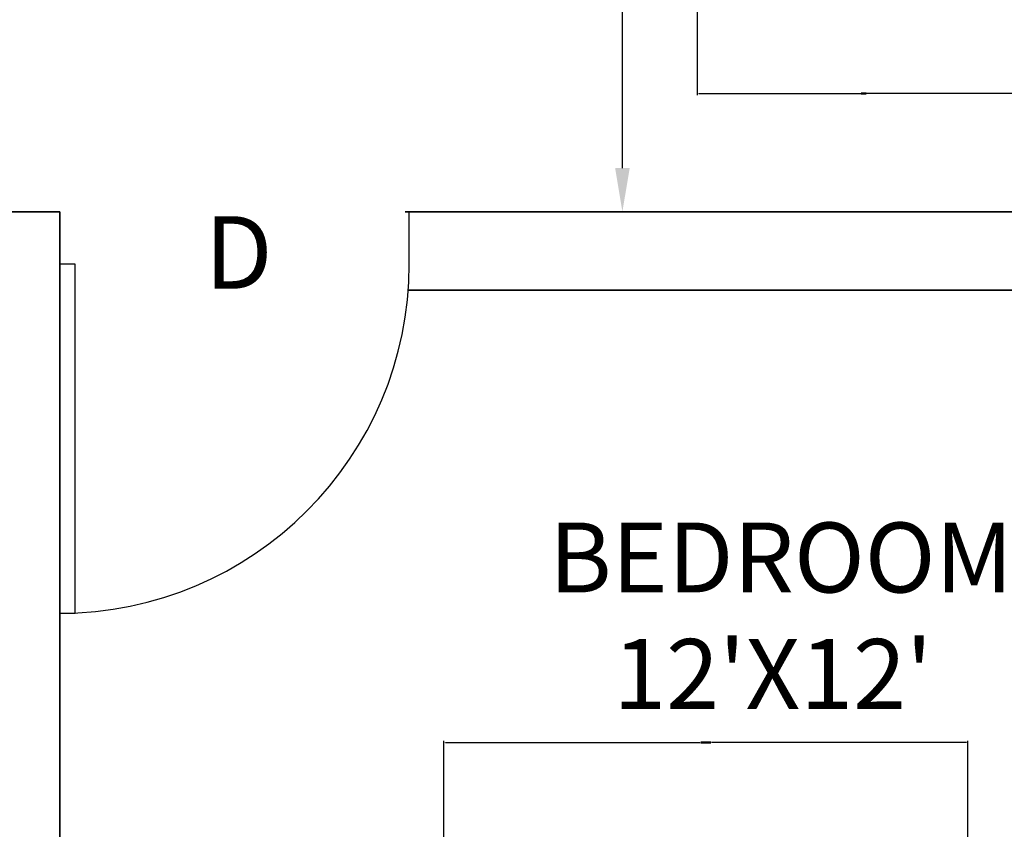
# Model space of a CAD drawing. Units: inches. Extents: x -128 to 854, y -395 to 398.
# Tile 30 of 61: x 152 to 265, y 2 to 95. Entities that reach past the tile are written whole.
import ezdxf

# ---------------------------------------------------------------- set-up
doc = ezdxf.new("R2010")
doc.units = ezdxf.units.IN
doc.header["$MEASUREMENT"] = 0
for name, color, linetype, lineweight in [('A-ANNO-DIMS', 2, 'Continuous', 18), ('A-ANNO-TEXT', 2, 'Continuous', 18), ('A-AREA-IDEN', 1, 'Continuous', 18), ('A-DOOR', 4, 'Continuous', 25), ('A-WALL', 4, 'Continuous', 35)]:
    doc.layers.add(name, color=color, linetype=linetype, lineweight=lineweight)
doc.styles.get("Standard").update_dxf_attribs({"font": 'arial.ttf'})
doc.dimstyles.get("Standard").update_dxf_attribs({"dimtxt": 0.18, "dimasz": 0.18, "dimexe": 0.18, "dimexo": 0.0625, "dimgap": 0.09, "dimtad": 0, "dimtih": 1, "dimtoh": 1, "dimdec": 1, "dimzin": 0, "dimdsep": 46, "dimlunit": 4, "dimtxsty": 'Standard', "dimcen": 0.09, "dimclrd": 1, "dimclre": 2, "dimclrt": 6, "dimadec": 0, "dimazin": 0, "dimtfac": 1, "dimtdec": 1, "dimtofl": 0, "dimtmove": 0, "dimatfit": 3, "dimfxl": 1, "dimtfill": 2, "dimtfillclr": 3, "dimtolj": 1, "dimtzin": 0, "dimarcsym": 0})

# ---------------------------------------------------------------- blocks, each defined once
blk = doc.blocks.new('*U9')
for p, q in [((0, 0), (0, 6)), ((40, 0), (40, 6))]:
    blk.add_line(p, q)
blk.add_lwpolyline([(0, 0), (0, -40), (1.75, -40), (1.75, 0)], close=True)
blk.add_arc((0, 0), 40, 270, 360)
blk = doc.blocks.new('*D55')
at = {"layer": 'A-ANNO-DIMS', "color": 0, "lineweight": -2, "transparency": 16777216}
for p, q in [((304.81, 186.74), (221.09, 186.74)), ((221.27, 181.74), (221.27, 131.87)), ((221.27, 77.74), (221.27, 127.61)), ((304.81, 72.74), (221.09, 72.74))]:
    blk.add_line(p, q, dxfattribs=at)
at = {"layer": 'A-ANNO-DIMS', "color": 0, "transparency": 16777216}
for points in [[(220.44, 181.74), (222.11, 181.74), (221.27, 186.74)], [(220.44, 77.74), (222.11, 77.74), (221.27, 72.74)]]:
    blk.add_solid(points, dxfattribs=at)
at = {"layer": 'Defpoints', "color": 0, "transparency": 16777216}
for p in [(221.27, 186.74), (304.87, 186.74), (304.87, 72.74)]:
    blk.add_point(p, dxfattribs=at)
at = {"layer": 'A-ANNO-DIMS', "color": 0, "transparency": 16777216, "insert": (221.27, 129.74), "char_height": 4, "attachment_point": 5, "bg_fill": 1, "box_fill_scale": 1.25, "bg_fill_color": 3, "bg_fill_transparency": 0}
blk.add_mtext('\\A1;9\'-6"', dxfattribs=at)
blk = doc.blocks.new('*D78')
at = {"layer": 'A-ANNO-DIMS', "color": 2, "lineweight": -2, "transparency": 16777216}
for p, q in [((200.83, 0.01), (200.83, 12.12)), ((260.83, 0.01), (260.83, 12.12))]:
    blk.add_line(p, q, dxfattribs=at)
at = {"layer": 'A-ANNO-DIMS', "color": 1, "lineweight": -2, "transparency": 16777216}
for p, q in [((201.01, 11.94), (230.19, 11.94)), ((260.65, 11.94), (231.47, 11.94))]:
    blk.add_line(p, q, dxfattribs=at)
at = {"layer": 'A-ANNO-DIMS', "color": 1, "transparency": 16777216}
for points in [[(201.01, 11.97), (201.01, 11.91), (200.83, 11.94)], [(260.65, 11.97), (260.65, 11.91), (260.83, 11.94)]]:
    blk.add_solid(points, dxfattribs=at)
at = {"layer": 'Defpoints', "color": 0, "transparency": 16777216}
for p in [(200.83, 11.94), (200.83, -0.06), (260.83, -0.06)]:
    blk.add_point(p, dxfattribs=at)
at = {"layer": 'A-ANNO-DIMS', "color": 6, "transparency": 16777216, "insert": (230.83, 11.94), "char_height": 0.18, "attachment_point": 5, "bg_fill": 1, "box_fill_scale": 1.25, "bg_fill_color": 3, "bg_fill_transparency": 0}
blk.add_mtext('\\A1;5\'-0" TYP.', dxfattribs=at)
blk = doc.blocks.new('*D92')
at = {"layer": 'A-ANNO-DIMS', "color": 2, "lineweight": -2, "transparency": 16777216}
for p, q in [((229.83, 95.67), (229.83, 86.09)), ((267.95, 95.67), (267.95, 86.09))]:
    blk.add_line(p, q, dxfattribs=at)
at = {"layer": 'A-ANNO-DIMS', "color": 1, "lineweight": -2, "transparency": 16777216}
for p, q in [((230.01, 86.27), (248.56, 86.27)), ((267.77, 86.27), (249.22, 86.27))]:
    blk.add_line(p, q, dxfattribs=at)
at = {"layer": 'A-ANNO-DIMS', "color": 1, "transparency": 16777216}
for points in [[(230.01, 86.3), (230.01, 86.24), (229.83, 86.27)], [(267.77, 86.3), (267.77, 86.24), (267.95, 86.27)]]:
    blk.add_solid(points, dxfattribs=at)
at = {"layer": 'Defpoints', "color": 0, "transparency": 16777216}
for p in [(229.83, 95.73), (267.95, 95.73), (267.95, 86.27)]:
    blk.add_point(p, dxfattribs=at)
at = {"layer": 'A-ANNO-DIMS', "color": 6, "transparency": 16777216, "insert": (248.89, 86.27), "char_height": 0.18, "attachment_point": 5, "bg_fill": 1, "box_fill_scale": 1.25, "bg_fill_color": 3, "bg_fill_transparency": 0}
blk.add_mtext('\\A1;3\'-2"', dxfattribs=at)

msp = doc.modelspace()

# ---------------------------------------------------------------- linework, layer by layer
at = {"layer": 'A-WALL'}
for p, q in [((156.87, 72.74), (147.87, 72.74)), ((156.87, 72.74), (156.87, -80.26)), ((304.87, 72.74), (196.42, 72.74)), ((304.87, 63.74), (196.76, 63.74))]:
    msp.add_line(p, q, dxfattribs=at)

# ---------------------------------------------------------------- block references
at = {"layer": 'A-DOOR'}
msp.add_blockref('*U9', (156.87, 66.74), dxfattribs=at)

# ---------------------------------------------------------------- texts
at = {"layer": 'A-ANNO-TEXT'}
msp.add_text('D', height=8.31, dxfattribs=at).set_placement((173.44, 63.91))
at = {"layer": 'A-AREA-IDEN', "insert": (212.88, 37.12), "char_height": 8, "attachment_point": 1}
msp.add_mtext_dynamic_manual_height_columns("BEDROOM\\P   12'X12'", width=99.0352, gutter_width=1, heights=[0], dxfattribs=at)

# ---------------------------------------------------------------- dimensions: what is measured, and where the dimension line sits
at = {"layer": 'A-ANNO-DIMS'}
dim = msp.add_linear_dim(base=(221.27, 186.74), p1=(304.87, 72.74), p2=(304.87, 186.74), angle=90, dimstyle='Standard', override={"dimtxt": 4, "dimasz": 5, "dimclrd": 0, "dimclre": 0, "dimclrt": 0}, dxfattribs=at)
dim.commit()
dim.dimension.update_dxf_attribs({"geometry": '*D55', "text_midpoint": (221.27, 129.74)})
dim = msp.add_linear_dim(base=(267.95, 86.27), p1=(229.83, 95.73), p2=(267.95, 95.73), dimstyle='Standard', override={"dimdec": 1, "dimlfac": 1, "dimrnd": 0, "dimzin": 1, "dimdsep": 46, "dimlunit": 4, "dimfrac": 2}, dxfattribs=at)
dim.commit()
dim.dimension.update_dxf_attribs({"geometry": '*D92', "text_midpoint": (248.89, 86.27)})
dim = msp.add_linear_dim(base=(200.83, 11.94), p1=(260.83, -0.06), p2=(200.83, -0.06), angle=180, text='<> TYP.', dimstyle='Standard', override={"dimdec": 1, "dimlfac": 1, "dimrnd": 0, "dimzin": 1, "dimdsep": 46, "dimlunit": 4, "dimfrac": 2}, dxfattribs=at)
dim.commit()
dim.dimension.update_dxf_attribs({"geometry": '*D78', "text_midpoint": (230.83, 11.94)})

doc.saveas('drawing.dxf')
